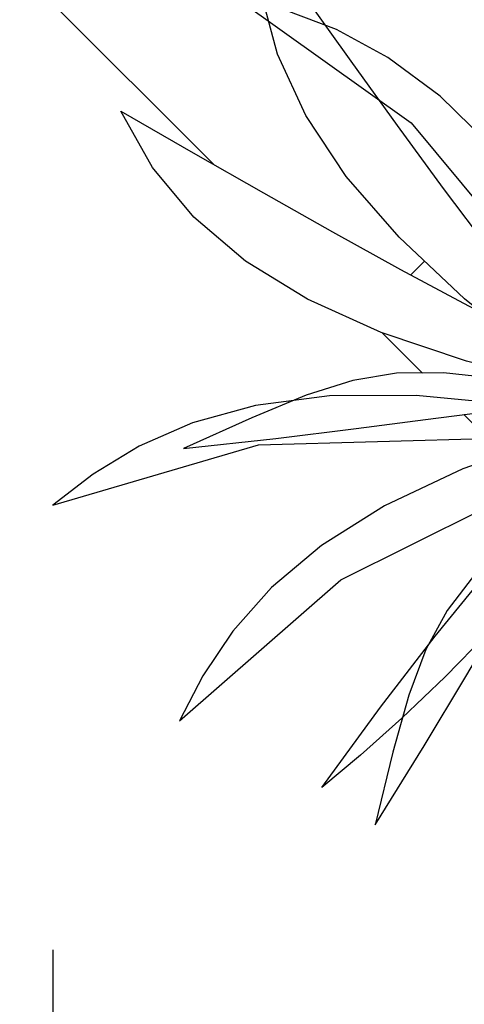
# Model space of a CAD drawing. Units: inches. Extents: x 3590 to 5167, y 65 to 1917.
# Tile 72 of 100: x 5035 to 5046, y 1765 to 1789. Entities that reach past the tile are written whole.
import ezdxf

# ---------------------------------------------------------------- set-up
doc = ezdxf.new("R2010")
doc.units = ezdxf.units.IN
for name, color, linetype, lineweight in [('A-ANNO-DIMS', 2, 'Continuous', 18), ('A-FLOR-PATT', 8, 'Continuous', 13), ('L-PLNT', 94, 'Continuous', 18)]:
    doc.layers.add(name, color=color, linetype=linetype, lineweight=lineweight)
doc.layers.add('DIENHOA', color=3, linetype='Continuous')
doc.styles.get("Standard").update_dxf_attribs({"font": 'arial.ttf'})
doc.dimstyles.new('ISO-25', dxfattribs={"dimtxt": 9, "dimasz": 2.5, "dimexe": 1.25, "dimexo": 0.625, "dimtad": 1, "dimdec": 1, "dimlunit": 3, "dimtxsty": 'Standard', "dimcen": 2.5, "dimadec": 0, "dimazin": 0, "dimtfac": 1, "dimtdec": 1, "dimtmove": 0, "dimatfit": 3, "dimfxl": 1, "dimarcsym": 0})

# ---------------------------------------------------------------- blocks, each defined once
blk = doc.blocks.new('Cay03_mb')
at = {"layer": 'DIENHOA'}
for p, q in [((-414.37, 402.78), (-240.22, 277.83)), ((-314.87, 371.26), (-365.2, 390.27)), ((-263.5, 343.48), (-314.87, 371.26)), ((-211.19, 304.6), (-263.5, 343.48)), ((-158.04, 252.34), (-211.19, 304.6)), ((-240.22, 277.83), (-88.39, 94.86)), ((-298.56, 20.07), (-345.02, 5.4)), ((-254.73, 27.37), (-298.56, 20.07)), ((-207.96, 27.76), (-254.73, 27.37)), ((-152.72, 21.72), (-207.96, 27.76)), ((-345.02, 5.4), (-399.63, -17.11)), ((-399.63, -17.11), (-467.96, -47.94)), ((-295.34, -27.91), (-225.83, -18.85)), ((-225.83, -18.85), (-165.8, -11.26)), ((-375.62, -37.81), (-295.34, -27.91)), ((-467.96, -47.94), (-375.62, -37.81)), ((-216.28, -235.58), (-165.86, -174.12)), ((-270.99, -306.55), (-216.28, -235.58)), ((-162.07, -230.91), (-206.29, -276.49)), ((-206.29, -276.49), (-249.56, -317.79)), ((-329.53, -387.1), (-270.99, -306.55)), ((-249.56, -317.79), (-290.96, -354.69)), ((-290.96, -354.69), (-329.53, -387.1))]:
    blk.add_line(p, q, dxfattribs=at)
for points in [[(-395.6, 473.65), (-347.51, 405.62), (-300.58, 339.5), (-254.33, 275.13), (-208.27, 212.32), (-161.92, 150.91), (-114.81, 90.72), (-66.46, 31.56), (-16.39, -26.73)], [(-16.39, -26.73), (-108.35, 38.55), (-186.88, 101.73), (-252.35, 163.45), (-305.09, 224.39), (-345.44, 285.22), (-373.75, 346.59), (-390.35, 409.18), (-395.6, 473.65)], [(-530.47, 289.69), (-458.27, 248.1), (-387.93, 207.77), (-318.94, 168.75), (-250.78, 131.06), (-182.94, 94.76), (-114.93, 59.88), (-46.22, 26.47), (23.69, -5.44)], [(23.69, -5.44), (-87.17, 15.25), (-184.97, 39.64), (-270.29, 68.2), (-343.73, 101.4), (-405.88, 139.68), (-457.33, 183.51), (-498.66, 233.36), (-530.47, 289.69)], [(-16.39, -26.73), (-133.98, -4.68), (-235.26, 5.29), (-321.98, 4.67), (-395.89, -5.03), (-458.73, -22.31), (-512.26, -45.67), (-558.22, -73.63), (-598.36, -104.66)], [(-471.89, -320.34), (-310.46, -179.32), (-97.66, -73.3), (23.69, -5.44)], [(23.69, -5.44), (-92.3, -34.76), (-188.42, -68.2), (-266.88, -105.14), (-329.9, -144.95), (-379.7, -187), (-418.48, -230.67), (-448.47, -275.32), (-471.89, -320.34)], [(-598.36, -104.66), (-392.67, -44.38), (-155.01, -37.42), (-16.39, -26.73)], [(-276.22, -424.43), (-227.35, -345.43), (-185.71, -276.08), (-150.05, -215.74), (-119.06, -163.76), (-91.49, -119.51), (-66.04, -82.35), (-41.43, -51.64), (-16.39, -26.73)], [(-16.39, -26.73), (-84.88, -85.96), (-136.99, -133.15), (-175.77, -172.96), (-204.26, -210.05), (-225.5, -249.08), (-242.55, -294.71), (-258.44, -351.61), (-276.22, -424.43)]]:
    blk.add_lwpolyline(points, dxfattribs=at)
blk = doc.blocks.new('*D322')
at = {"layer": 'A-ANNO-DIMS', "color": 0, "lineweight": -2, "transparency": 16777216}
for p, q in [((5035.744, 1766.184), (5035.744, 1761.199)), ((5064.812, 1766.184), (5064.812, 1761.199)), ((5038.244, 1762.449), (5062.312, 1762.449)), ((5064.812, 1762.449), (5166.991, 1762.449))]:
    blk.add_line(p, q, dxfattribs=at)
at = {"layer": 'A-ANNO-DIMS', "color": 0, "transparency": 16777216}
for points in [[(5038.244, 1762.866), (5038.244, 1762.032), (5035.744, 1762.449)], [(5062.312, 1762.866), (5062.312, 1762.032), (5064.812, 1762.449)]]:
    blk.add_solid(points, dxfattribs=at)
at = {"layer": 'Defpoints', "color": 0, "transparency": 16777216}
for p in [(5035.744, 1766.809), (5064.812, 1766.809), (5064.812, 1762.449)]:
    blk.add_point(p, dxfattribs=at)
at = {"layer": 'A-ANNO-DIMS', "color": 0, "transparency": 16777216, "insert": (5117.152, 1767.669), "char_height": 9, "attachment_point": 5}
blk.add_mtext('PLANT 2\'-5" TYP.', dxfattribs=at)
blk = doc.blocks.new('*D323')
at = {"layer": 'A-ANNO-DIMS', "color": 0, "lineweight": -2, "transparency": 16777216}
for p, q in [((5069.172, 1795.216), (5069.172, 1874.95)), ((5065.437, 1795.216), (5070.422, 1795.216)), ((5069.172, 1769.309), (5069.172, 1792.716)), ((5065.437, 1766.809), (5070.422, 1766.809))]:
    blk.add_line(p, q, dxfattribs=at)
at = {"layer": 'A-ANNO-DIMS', "color": 0, "transparency": 16777216}
for points in [[(5068.756, 1792.716), (5069.589, 1792.716), (5069.172, 1795.216)], [(5068.756, 1769.309), (5069.589, 1769.309), (5069.172, 1766.809)]]:
    blk.add_solid(points, dxfattribs=at)
at = {"layer": 'Defpoints', "color": 0, "transparency": 16777216}
for p in [(5064.812, 1795.216), (5069.172, 1795.216), (5064.812, 1766.809)]:
    blk.add_point(p, dxfattribs=at)
at = {"layer": 'A-ANNO-DIMS', "color": 0, "transparency": 16777216, "insert": (5063.894, 1836.333), "char_height": 9, "attachment_point": 5, "rotation": 90}
blk.add_mtext('2\'-4 1/2" TYP.', dxfattribs=at)

msp = doc.modelspace()

# ---------------------------------------------------------------- hatches: boundary and pattern name
at = {"layer": 'A-FLOR-PATT', "transparency": 33554687}
h = msp.add_hatch(dxfattribs=at)
h.set_pattern_fill('AR-HBONE', color=256, scale=0.2)
h.set_pattern_definition([(45, (-588.972, 0), (0, 28.73682), [60.96, -20.32]), (135, (-574.604, 14.368), (3e-15, 28.73682), [60.96, -20.32])])
h.paths.add_polyline_path([(5071.274, 1796.999), (4933.274, 1796.999), (4933.274, 1753.999), (4962.774, 1753.999, -0.414214), (4928.774, 1719.999), (4933.274, 1718.999), (4933.274, 1334.999), (5071.274, 1334.999)])
h.paths.add_polyline_path([(4951.78, 1521.077), (4951.715, 1521.04), (4951.563, 1520.895)], flags=16)
h.paths.add_polyline_path([(4952.267, 1521.376), (4952.198, 1521.371), (4952.198, 1521.356)], flags=0)
h.paths.add_polyline_path([(4967.051, 1529.728), (4965.231, 1528.694), (4963.411, 1527.714), (4961.756, 1526.851), (4963.589, 1527.449), (4964.036, 1527.478), (4962.975, 1527.249), (4961.76, 1526.852), (4959.792, 1525.834), (4958.005, 1524.895), (4956.24, 1523.93), (4954.504, 1522.919), (4954.129, 1522.682), (4953.361, 1521.997), (4953.366, 1521.998), (4953.605, 1522.064), (4955.106, 1522.761), (4956.921, 1523.434), (4958.678, 1523.915), (4960.358, 1524.2), (4961.945, 1524.286), (4964.171, 1524.108), (4965.958, 1523.309), (4963.863, 1522.976), (4965.187, 1522.499), (4963.366, 1522.497), (4961.545, 1522.487), (4959.764, 1522.461), (4958.304, 1522.419), (4957.974, 1522.388), (4956.307, 1522.232), (4954.718, 1522.071), (4953.251, 1521.899), (4953.525, 1521.623), (4954.331, 1521.379), (4956.243, 1521.23), (4958.039, 1520.93), (4959.684, 1520.483), (4961.16, 1519.896), (4963.107, 1518.8), (4964.393, 1517.325), (4962.973, 1517.726), (4964.558, 1516.661), (4965.407, 1515.708), (4963.507, 1516.322), (4961.68, 1517.005), (4959.935, 1517.745), (4958.282, 1518.528), (4956.732, 1519.343), (4955.295, 1520.175), (4954.672, 1520.572), (4954.513, 1520.627), (4955.658, 1519.318), (4956.703, 1517.982), (4957.644, 1516.647), (4958.485, 1515.334), (4959.55, 1513.524), (4960.438, 1511.769), (4958.841, 1513.62), (4957.452, 1515.325), (4955.819, 1517.459), (4956.665, 1515.448), (4957.111, 1513.923), (4957.447, 1511.714), (4957.076, 1509.793), (4956.538, 1511.11), (4955.992, 1512.569), (4955.444, 1514.125), (4954.898, 1515.735), (4954.357, 1517.356), (4953.824, 1518.943), (4953.305, 1520.452), (4953.065, 1521.116), (4952.971, 1521.146), (4952.949, 1521.086), (4952.73, 1520.199), (4953.37, 1518.024), (4953.757, 1516.373), (4954.051, 1514.765), (4954.264, 1513.221), (4954.471, 1511.131), (4954.497, 1510.402), (4954.409, 1511.76), (4954.264, 1513.221), (4954.051, 1514.765), (4953.757, 1516.373), (4953.37, 1518.024), (4952.877, 1519.698), (4952.716, 1520.141), (4952.533, 1519.059), (4952.374, 1517.789), (4952.219, 1516.312), (4952.046, 1514.6), (4951.833, 1512.626), (4951.557, 1510.363), (4951.203, 1512.168), (4950.852, 1514.339), (4950.985, 1516.376), (4951.66, 1518.286), (4952.593, 1520.481), (4952.357, 1521.13), (4951.855, 1520.328), (4950.839, 1518.908), (4949.777, 1517.587), (4948.916, 1516.617), (4948.111, 1515.256), (4947.089, 1513.554), (4945.889, 1511.615), (4946.326, 1513.402), (4946.562, 1514.249), (4945.528, 1513.327), (4944.581, 1512.531), (4946.018, 1514.508), (4947.204, 1516.048), (4947.893, 1517.313), (4949.307, 1518.764), (4950.414, 1519.767), (4950.451, 1519.806), (4952.267, 1521.376), (4951.645, 1521.493), (4950.404, 1521.18), (4948.044, 1520.359), (4946.119, 1519.452), (4944.572, 1518.475), (4943.35, 1517.443), (4941.997, 1515.92), (4941.661, 1515.275), (4942.813, 1516.99), (4944.572, 1518.475), (4946.119, 1519.452), (4948.044, 1520.359), (4950.404, 1521.18), (4951.645, 1521.493), (4949.647, 1521.868), (4948.6, 1521.756), (4947.126, 1521.57), (4945.42, 1521.348), (4943.45, 1521.105), (4941.183, 1520.856), (4942.86, 1521.613), (4943.873, 1522.03), (4942.952, 1521.909), (4941.41, 1521.485), (4939.543, 1520.67), (4938.968, 1520.226), (4940.733, 1521.299), (4942.952, 1521.909), (4943.702, 1522.008), (4945.894, 1522.7), (4947.565, 1522.714), (4948.921, 1522.566), (4951.131, 1522.183), (4950.971, 1522.297), (4948.129, 1523.006), (4946.035, 1523.707), (4944.232, 1524.521), (4942.707, 1525.461), (4941.444, 1526.537), (4940.43, 1527.761), (4939.649, 1529.143), (4941.421, 1528.122), (4943.147, 1527.132), (4944.841, 1526.175), (4946.514, 1525.25), (4948.179, 1524.359), (4948.365, 1524.263), (4946.475, 1526.045), (4945.181, 1527.54), (4944.19, 1529.033), (4943.496, 1530.54), (4943.278, 1531.36), (4942.498, 1531.919), (4943.114, 1531.762), (4942.959, 1533.659), (4944.14, 1531.989), (4944.612, 1531.323), (4946.202, 1530.463), (4947.486, 1529.509), (4948.79, 1528.226), (4950.368, 1526.237), (4949.485, 1528.155), (4948.851, 1530.123), (4948.491, 1532.041), (4948.381, 1533.918), (4948.501, 1535.76), (4948.827, 1537.573), (4949.418, 1535.565), (4949.957, 1533.569), (4950.464, 1531.586), (4950.961, 1529.617), (4951.391, 1527.954), (4951.724, 1530.687), (4952.201, 1532.58), (4952.889, 1534.33), (4953.77, 1535.951), (4954.827, 1537.46), (4954.521, 1535.39), (4954.273, 1533.937), (4955.58, 1535.663), (4956.748, 1536.739), (4956.159, 1534.78), (4955.589, 1532.873), (4955.043, 1531.006), (4954.525, 1529.166), (4954.038, 1527.341), (4953.638, 1525.733), (4953.611, 1525.586), (4953.398, 1524.166), (4953.382, 1524.009), (4954.07, 1525.476), (4954.912, 1527.022), (4956.136, 1528.894), (4957.847, 1530.577), (4959.376, 1531.54), (4958.256, 1530.104), (4957.143, 1528.663), (4956.066, 1527.243), (4955.056, 1525.871), (4954.141, 1524.571), (4953.352, 1523.372), (4953.311, 1523.303), (4953.273, 1522.925), (4953.261, 1522.382), (4954.103, 1523.373), (4954.63, 1524.284), (4955.961, 1526.358), (4957.23, 1528.13), (4958.421, 1529.609), (4960.037, 1531.368), (4961.374, 1532.375), (4962.101, 1532.77), (4961.07, 1531.061), (4959.987, 1529.438), (4958.869, 1527.908), (4958.15, 1527.007), (4959.803, 1528.003), (4961.589, 1528.793), (4963.391, 1529.328), (4965.211, 1529.632)], flags=16)
h.paths.add_polyline_path([(4962.944, 1523.182), (4961.107, 1523.422), (4960.392, 1523.362), (4962.35, 1523.331)], flags=0)
h.paths.add_polyline_path([(5049.541, 1584.551), (5049.476, 1584.515), (5049.325, 1584.37)], flags=16)
h.paths.add_polyline_path([(5050.028, 1584.851), (5049.959, 1584.845), (5049.959, 1584.83)], flags=0)
h.paths.add_polyline_path([(5042.333, 1581.949), (5043.88, 1582.926), (5045.806, 1583.833), (5048.165, 1584.654), (5049.406, 1584.967), (5047.408, 1585.342), (5046.361, 1585.231), (5044.888, 1585.044), (5043.181, 1584.822), (5041.211, 1584.579), (5038.944, 1584.33), (5040.622, 1585.087), (5041.634, 1585.504), (5040.713, 1585.383), (5039.171, 1584.959), (5037.304, 1584.144), (5036.729, 1583.7), (5038.494, 1584.773), (5040.713, 1585.383), (5041.463, 1585.482), (5043.655, 1586.174), (5045.326, 1586.188), (5046.682, 1586.04), (5048.893, 1585.657), (5048.732, 1585.771), (5045.891, 1586.48), (5043.796, 1587.181), (5041.994, 1587.996), (5040.468, 1588.935), (5039.205, 1590.011), (5038.191, 1591.235), (5037.41, 1592.617), (5039.182, 1591.596), (5040.909, 1590.607), (5042.602, 1589.649), (5044.275, 1588.724), (5045.94, 1587.833), (5046.126, 1587.738), (5044.237, 1589.519), (5042.942, 1591.015), (5041.952, 1592.508), (5041.257, 1594.014), (5041.039, 1594.834), (5040.26, 1595.393), (5040.875, 1595.237), (5040.721, 1597.133), (5041.901, 1595.463), (5042.373, 1594.798), (5043.963, 1593.938), (5045.247, 1592.983), (5046.552, 1591.701), (5048.129, 1589.712), (5047.247, 1591.63), (5046.613, 1593.597), (5046.252, 1595.515), (5046.142, 1597.392), (5046.262, 1599.234), (5046.588, 1601.047), (5047.179, 1599.039), (5047.718, 1597.043), (5048.225, 1595.06), (5048.722, 1593.091), (5049.152, 1591.429), (5049.485, 1594.161), (5049.962, 1596.054), (5050.65, 1597.804), (5051.532, 1599.425), (5052.589, 1600.934), (5052.283, 1598.864), (5052.034, 1597.411), (5053.341, 1599.137), (5054.509, 1600.213), (5053.92, 1598.254), (5053.35, 1596.348), (5052.805, 1594.48), (5052.286, 1592.64), (5051.799, 1590.815), (5051.4, 1589.207), (5051.373, 1589.06), (5051.159, 1587.64), (5051.143, 1587.483), (5051.831, 1588.95), (5052.673, 1590.496), (5053.898, 1592.368), (5055.608, 1594.051), (5057.137, 1595.014), (5056.017, 1593.578), (5054.904, 1592.137), (5053.828, 1590.717), (5052.817, 1589.345), (5051.902, 1588.046), (5051.113, 1586.846), (5051.072, 1586.777), (5051.034, 1586.399), (5051.022, 1585.856), (5051.864, 1586.847), (5052.391, 1587.758), (5053.723, 1589.832), (5054.991, 1591.604), (5056.182, 1593.083), (5057.798, 1594.842), (5059.135, 1595.849), (5059.863, 1596.244), (5058.831, 1594.535), (5057.749, 1592.912), (5056.63, 1591.382), (5055.912, 1590.482), (5057.564, 1591.477), (5059.35, 1592.267), (5061.152, 1592.802), (5062.972, 1593.106), (5064.812, 1593.203), (5062.992, 1592.169), (5061.172, 1591.188), (5059.518, 1590.325), (5061.35, 1590.924), (5061.797, 1590.952), (5060.737, 1590.723), (5059.521, 1590.326), (5057.553, 1589.308), (5055.766, 1588.369), (5054.002, 1587.404), (5052.265, 1586.393), (5051.891, 1586.156), (5051.122, 1585.471), (5051.127, 1585.472), (5051.366, 1585.538), (5052.867, 1586.235), (5054.682, 1586.908), (5056.439, 1587.389), (5058.12, 1587.675), (5059.706, 1587.76), (5061.933, 1587.583), (5063.719, 1586.783), (5061.624, 1586.45), (5062.949, 1585.973), (5061.127, 1585.971), (5059.307, 1585.961), (5057.525, 1585.935), (5056.065, 1585.893), (5055.735, 1585.862), (5054.068, 1585.707), (5052.479, 1585.546), (5051.012, 1585.373), (5051.286, 1585.097), (5052.092, 1584.853), (5054.004, 1584.704), (5055.8, 1584.404), (5057.446, 1583.958), (5058.921, 1583.37), (5060.868, 1582.274), (5062.154, 1580.799), (5060.734, 1581.2), (5062.32, 1580.135), (5063.168, 1579.182), (5061.269, 1579.796), (5059.441, 1580.479), (5057.696, 1581.219), (5056.043, 1582.003), (5054.493, 1582.817), (5053.057, 1583.649), (5052.433, 1584.047), (5052.274, 1584.101), (5053.42, 1582.793), (5054.464, 1581.457), (5055.405, 1580.121), (5056.247, 1578.809), (5057.311, 1576.998), (5058.199, 1575.244), (5056.602, 1577.094), (5055.213, 1578.799), (5053.58, 1580.933), (5054.427, 1578.922), (5054.872, 1577.397), (5055.208, 1575.189), (5054.838, 1573.267), (5054.299, 1574.584), (5053.754, 1576.043), (5053.206, 1577.599), (5052.659, 1579.209), (5052.118, 1580.83), (5051.585, 1582.417), (5051.066, 1583.927), (5050.826, 1584.59), (5050.733, 1584.62), (5050.711, 1584.561), (5050.491, 1583.673), (5051.131, 1581.498), (5051.518, 1579.847), (5051.813, 1578.24), (5052.026, 1576.695), (5052.233, 1574.605), (5052.258, 1573.876), (5052.17, 1575.234), (5052.026, 1576.695), (5051.813, 1578.24), (5051.518, 1579.847), (5051.131, 1581.498), (5050.638, 1583.172), (5050.477, 1583.615), (5050.294, 1582.533), (5050.136, 1581.263), (5049.981, 1579.786), (5049.807, 1578.074), (5049.594, 1576.1), (5049.318, 1573.837), (5048.965, 1575.642), (5048.613, 1577.813), (5048.747, 1579.85), (5049.421, 1581.76), (5050.354, 1583.955), (5050.118, 1584.604), (5049.616, 1583.802), (5048.6, 1582.382), (5047.538, 1581.061), (5046.677, 1580.091), (5045.872, 1578.73), (5044.85, 1577.028), (5043.651, 1575.089), (5044.087, 1576.877), (5044.324, 1577.723), (5043.289, 1576.801), (5042.342, 1576.005), (5043.779, 1577.982), (5044.966, 1579.522), (5045.655, 1580.787), (5047.068, 1582.239), (5048.175, 1583.241), (5048.213, 1583.28), (5050.028, 1584.851), (5049.406, 1584.967), (5048.165, 1584.654), (5045.806, 1583.833), (5043.88, 1582.926), (5042.333, 1581.949), (5041.111, 1580.917), (5039.758, 1579.394), (5039.423, 1578.749), (5040.575, 1580.464)], flags=16)
h.paths.add_polyline_path([(4954.799, 1533.12), (4954.262, 1532.079), (4953.831, 1530.935), (4953.505, 1529.636), (4953.283, 1528.133), (4953.167, 1526.376), (4953.156, 1524.315), (4953.277, 1521.236), (4952.802, 1521.842), (4951.557, 1521.998), (4950.976, 1521.961), (4952.661, 1521.941), (4952.802, 1521.842), (4953.152, 1523.593), (4953.167, 1526.376), (4953.283, 1528.133), (4953.609, 1530.346), (4954.456, 1532.592)], flags=0)
h.paths.add_polyline_path([(5050.563, 1585.316), (5049.318, 1585.472), (5048.737, 1585.435), (5050.422, 1585.415), (5050.563, 1585.316), (5050.914, 1587.067), (5050.928, 1589.851), (5051.045, 1591.607), (5051.371, 1593.82), (5052.217, 1596.066), (5052.56, 1596.594), (5052.024, 1595.554), (5051.592, 1594.409), (5051.266, 1593.11), (5051.045, 1591.607), (5050.928, 1589.851), (5050.918, 1587.789), (5051.038, 1584.71)], flags=0)
h.paths.add_polyline_path([(5058.153, 1586.836), (5060.111, 1586.805), (5060.705, 1586.656), (5058.868, 1586.896)], flags=0)
h.paths.add_polyline_path([(5049.541, 1430.936), (5049.476, 1430.9), (5049.325, 1430.755)], flags=16)
h.paths.add_polyline_path([(5050.028, 1431.236), (5049.959, 1431.231), (5049.959, 1431.215)], flags=0)
h.paths.add_polyline_path([(5046.588, 1447.432), (5047.179, 1445.425), (5047.718, 1443.429), (5048.225, 1441.446), (5048.722, 1439.476), (5049.152, 1437.814), (5049.485, 1440.546), (5049.962, 1442.439), (5050.65, 1444.189), (5051.532, 1445.811), (5052.589, 1447.319), (5052.283, 1445.249), (5052.034, 1443.796), (5053.341, 1445.522), (5054.509, 1446.598), (5053.92, 1444.64), (5053.35, 1442.733), (5052.805, 1440.865), (5052.286, 1439.025), (5051.799, 1437.201), (5051.4, 1435.592), (5051.373, 1435.445), (5051.159, 1434.025), (5051.143, 1433.868), (5051.831, 1435.335), (5052.673, 1436.881), (5053.898, 1438.753), (5055.608, 1440.436), (5057.137, 1441.4), (5056.017, 1439.963), (5054.904, 1438.522), (5053.828, 1437.102), (5052.817, 1435.73), (5051.902, 1434.431), (5051.113, 1433.231), (5051.072, 1433.162), (5051.034, 1432.784), (5051.022, 1432.242), (5051.864, 1433.232), (5052.391, 1434.143), (5053.723, 1436.217), (5054.991, 1437.989), (5056.182, 1439.468), (5057.798, 1441.227), (5059.135, 1442.235), (5059.863, 1442.629), (5058.831, 1440.921), (5057.749, 1439.298), (5056.63, 1437.767), (5055.912, 1436.867), (5057.564, 1437.863), (5059.35, 1438.652), (5061.152, 1439.187), (5062.972, 1439.491), (5064.812, 1439.588), (5062.992, 1438.554), (5061.172, 1437.573), (5059.518, 1436.71), (5061.35, 1437.309), (5061.797, 1437.337), (5060.737, 1437.108), (5059.521, 1436.711), (5057.553, 1435.693), (5055.766, 1434.754), (5054.002, 1433.789), (5052.265, 1432.778), (5051.891, 1432.541), (5051.122, 1431.856), (5051.127, 1431.857), (5051.366, 1431.923), (5052.867, 1432.62), (5054.682, 1433.293), (5056.439, 1433.775), (5058.12, 1434.06), (5059.706, 1434.145), (5061.933, 1433.968), (5063.719, 1433.168), (5061.624, 1432.835), (5062.949, 1432.358), (5061.127, 1432.357), (5059.307, 1432.346), (5057.525, 1432.32), (5056.065, 1432.278), (5055.735, 1432.248), (5054.068, 1432.092), (5052.479, 1431.931), (5051.012, 1431.759), (5051.286, 1431.482), (5052.092, 1431.238), (5054.004, 1431.089), (5055.8, 1430.789), (5057.446, 1430.343), (5058.921, 1429.755), (5060.868, 1428.66), (5062.154, 1427.185), (5060.734, 1427.585), (5062.32, 1426.52), (5063.168, 1425.567), (5061.269, 1426.181), (5059.441, 1426.865), (5057.696, 1427.604), (5056.043, 1428.388), (5054.493, 1429.202), (5053.057, 1430.034), (5052.433, 1430.432), (5052.274, 1430.487), (5053.42, 1429.178), (5054.464, 1427.842), (5055.405, 1426.506), (5056.247, 1425.194), (5057.311, 1423.383), (5058.199, 1421.629), (5056.602, 1423.479), (5055.213, 1425.184), (5053.58, 1427.318), (5054.427, 1425.307), (5054.872, 1423.782), (5055.208, 1421.574), (5054.838, 1419.652), (5054.299, 1420.97), (5053.754, 1422.428), (5053.206, 1423.984), (5052.659, 1425.595), (5052.118, 1427.215), (5051.585, 1428.802), (5051.066, 1430.312), (5050.826, 1430.975), (5050.733, 1431.005), (5050.711, 1430.946), (5050.491, 1430.058), (5051.131, 1427.883), (5051.518, 1426.232), (5051.813, 1424.625), (5052.026, 1423.081), (5052.233, 1420.991), (5052.258, 1420.261), (5052.17, 1421.619), (5052.026, 1423.081), (5051.813, 1424.625), (5051.518, 1426.232), (5051.131, 1427.883), (5050.638, 1429.558), (5050.477, 1430.001), (5050.294, 1428.918), (5050.136, 1427.648), (5049.981, 1426.171), (5049.807, 1424.459), (5049.594, 1422.485), (5049.318, 1420.222), (5048.965, 1422.028), (5048.613, 1424.199), (5048.747, 1426.235), (5049.421, 1428.146), (5050.354, 1430.34), (5050.118, 1430.989), (5049.616, 1430.187), (5048.6, 1428.768), (5047.538, 1427.446), (5046.677, 1426.477), (5045.872, 1425.116), (5044.85, 1423.413), (5043.651, 1421.474), (5044.087, 1423.262), (5044.324, 1424.109), (5043.289, 1423.186), (5042.342, 1422.391), (5043.779, 1424.368), (5044.966, 1425.907), (5045.655, 1427.173), (5047.068, 1428.624), (5048.175, 1429.627), (5048.213, 1429.666), (5050.028, 1431.236), (5049.406, 1431.353), (5048.165, 1431.039), (5045.806, 1430.218), (5043.88, 1429.311), (5042.333, 1428.334), (5041.111, 1427.302), (5039.758, 1425.779), (5039.423, 1425.134), (5040.575, 1426.849), (5042.333, 1428.334), (5043.88, 1429.311), (5045.806, 1430.218), (5048.165, 1431.039), (5049.406, 1431.353), (5047.408, 1431.727), (5046.361, 1431.616), (5044.888, 1431.429), (5043.181, 1431.207), (5041.211, 1430.964), (5038.944, 1430.715), (5040.622, 1431.472), (5041.634, 1431.89), (5040.713, 1431.769), (5039.171, 1431.345), (5037.304, 1430.53), (5036.729, 1430.085), (5038.494, 1431.158), (5040.713, 1431.769), (5041.463, 1431.867), (5043.655, 1432.559), (5045.326, 1432.573), (5046.682, 1432.425), (5048.893, 1432.042), (5048.732, 1432.156), (5045.891, 1432.865), (5043.796, 1433.566), (5041.994, 1434.381), (5040.468, 1435.321), (5039.205, 1436.396), (5038.191, 1437.62), (5037.41, 1439.002), (5039.182, 1437.982), (5040.909, 1436.992), (5042.602, 1436.034), (5044.275, 1435.109), (5045.94, 1434.218), (5046.126, 1434.123), (5044.237, 1435.904), (5042.942, 1437.4), (5041.952, 1438.893), (5041.257, 1440.399), (5041.039, 1441.219), (5040.26, 1441.778), (5040.875, 1441.622), (5040.721, 1443.518), (5041.901, 1441.848), (5042.373, 1441.183), (5043.963, 1440.323), (5045.247, 1439.369), (5046.552, 1438.086), (5048.129, 1436.097), (5047.247, 1438.015), (5046.613, 1439.982), (5046.252, 1441.901), (5046.142, 1443.778), (5046.262, 1445.619)], flags=16)
h.paths.add_polyline_path([(5052.382, 1444.255), (5051.623, 1442.78), (5052.024, 1441.939), (5052.56, 1442.98)], flags=0)
h.paths.add_polyline_path([(5050.563, 1431.701), (5049.318, 1431.857), (5048.737, 1431.821), (5050.422, 1431.8)], flags=0)
h.paths.add_polyline_path([(5058.153, 1433.221), (5060.111, 1433.19), (5060.705, 1433.041), (5058.868, 1433.281)], flags=0)
h.paths.add_polyline_path([(5049.541, 1352.285), (5049.476, 1352.249), (5049.325, 1352.104)], flags=16)
h.paths.add_polyline_path([(5050.028, 1352.585), (5049.959, 1352.58), (5049.959, 1352.564)], flags=0)
h.paths.add_polyline_path([(5046.588, 1368.781), (5047.179, 1366.774), (5047.718, 1364.778), (5048.225, 1362.795), (5048.722, 1360.825), (5049.152, 1359.163), (5049.485, 1361.896), (5049.962, 1363.789), (5050.65, 1365.538), (5051.532, 1367.16), (5052.589, 1368.669), (5052.283, 1366.598), (5052.034, 1365.145), (5053.341, 1366.871), (5054.509, 1367.947), (5053.92, 1365.989), (5053.35, 1364.082), (5052.805, 1362.214), (5052.286, 1360.374), (5051.799, 1358.55), (5051.4, 1356.942), (5051.373, 1356.794), (5051.159, 1355.374), (5051.143, 1355.218), (5051.831, 1356.684), (5052.673, 1358.23), (5053.898, 1360.102), (5055.608, 1361.786), (5057.137, 1362.749), (5056.017, 1361.313), (5054.904, 1359.872), (5053.828, 1358.452), (5052.817, 1357.079), (5051.902, 1355.78), (5051.113, 1354.581), (5051.072, 1354.512), (5051.034, 1354.133), (5051.022, 1353.591), (5051.864, 1354.581), (5052.391, 1355.492), (5053.723, 1357.566), (5054.991, 1359.338), (5056.182, 1360.817), (5057.798, 1362.577), (5059.135, 1363.584), (5059.863, 1363.979), (5058.831, 1362.27), (5057.749, 1360.647), (5056.63, 1359.117), (5055.912, 1358.216), (5057.564, 1359.212), (5059.35, 1360.001), (5061.152, 1360.536), (5062.972, 1360.841), (5064.812, 1360.937), (5062.992, 1359.903), (5061.172, 1358.923), (5059.518, 1358.059), (5061.35, 1358.658), (5061.797, 1358.687), (5060.737, 1358.458), (5059.521, 1358.061), (5057.553, 1357.043), (5055.766, 1356.103), (5054.002, 1355.138), (5052.265, 1354.127), (5051.891, 1353.89), (5051.122, 1353.206), (5051.127, 1353.206), (5051.366, 1353.272), (5052.867, 1353.969), (5054.682, 1354.643), (5056.439, 1355.124), (5058.12, 1355.409), (5059.706, 1355.495), (5061.933, 1355.317), (5063.719, 1354.518), (5061.624, 1354.184), (5062.949, 1353.708), (5061.127, 1353.706), (5059.307, 1353.695), (5057.525, 1353.669), (5056.065, 1353.627), (5055.735, 1353.597), (5054.068, 1353.441), (5052.479, 1353.28), (5051.012, 1353.108), (5051.286, 1352.831), (5052.092, 1352.587), (5054.004, 1352.439), (5055.8, 1352.138), (5057.446, 1351.692), (5058.921, 1351.104), (5060.868, 1350.009), (5062.154, 1348.534), (5060.734, 1348.935), (5062.32, 1347.869), (5063.168, 1346.916), (5061.269, 1347.53), (5059.441, 1348.214), (5057.696, 1348.954), (5056.043, 1349.737), (5054.493, 1350.551), (5053.057, 1351.383), (5052.433, 1351.781), (5052.274, 1351.836), (5053.42, 1350.527), (5054.464, 1349.191), (5055.405, 1347.855), (5056.247, 1346.543), (5057.311, 1344.733), (5058.199, 1342.978), (5056.602, 1344.828), (5055.213, 1346.534), (5053.58, 1348.667), (5054.427, 1346.656), (5054.872, 1345.132), (5055.208, 1342.923), (5054.838, 1341.002), (5054.299, 1342.319), (5053.754, 1343.778), (5053.206, 1345.334), (5052.659, 1346.944), (5052.118, 1348.564), (5051.585, 1350.151), (5051.066, 1351.661), (5050.826, 1352.324), (5050.733, 1352.355), (5050.711, 1352.295), (5050.491, 1351.408), (5051.131, 1349.232), (5051.518, 1347.581), (5051.813, 1345.974), (5052.026, 1344.43), (5052.233, 1342.34), (5052.258, 1341.61), (5052.17, 1342.969), (5052.026, 1344.43), (5051.813, 1345.974), (5051.518, 1347.581), (5051.131, 1349.232), (5050.638, 1350.907), (5050.477, 1351.35), (5050.294, 1350.267), (5050.136, 1348.997), (5049.981, 1347.52), (5049.807, 1345.809), (5049.594, 1343.835), (5049.318, 1341.571), (5048.965, 1343.377), (5048.613, 1345.548), (5048.747, 1347.585), (5049.421, 1349.495), (5050.354, 1351.689), (5050.118, 1352.339), (5049.616, 1351.536), (5048.6, 1350.117), (5047.538, 1348.795), (5046.677, 1347.826), (5045.872, 1346.465), (5044.85, 1344.763), (5043.651, 1342.824), (5044.087, 1344.611), (5044.324, 1345.458), (5043.289, 1344.535), (5042.342, 1343.74), (5043.779, 1345.717), (5044.966, 1347.256), (5045.655, 1348.522), (5047.068, 1349.973), (5048.175, 1350.976), (5048.213, 1351.015), (5050.028, 1352.585), (5049.406, 1352.702), (5048.165, 1352.388), (5045.806, 1351.567), (5043.88, 1350.661), (5042.333, 1349.683), (5041.111, 1348.651), (5039.758, 1347.128), (5039.423, 1346.483), (5040.575, 1348.198), (5042.333, 1349.683), (5043.88, 1350.661), (5045.806, 1351.567), (5048.165, 1352.388), (5049.406, 1352.702), (5047.408, 1353.076), (5046.361, 1352.965), (5044.888, 1352.779), (5043.181, 1352.556), (5041.211, 1352.313), (5038.944, 1352.065), (5040.622, 1352.821), (5041.634, 1353.239), (5040.713, 1353.118), (5039.171, 1352.694), (5037.304, 1351.879), (5036.729, 1351.434), (5038.494, 1352.508), (5040.713, 1353.118), (5041.463, 1353.216), (5043.655, 1353.909), (5045.326, 1353.923), (5046.682, 1353.774), (5048.893, 1353.391), (5048.732, 1353.506), (5045.891, 1354.214), (5043.796, 1354.915), (5041.994, 1355.73), (5040.468, 1356.67), (5039.205, 1357.746), (5038.191, 1358.969), (5037.41, 1360.352), (5039.182, 1359.331), (5040.909, 1358.341), (5042.602, 1357.383), (5044.275, 1356.458), (5045.94, 1355.567), (5046.126, 1355.472), (5044.237, 1357.253), (5042.942, 1358.749), (5041.952, 1360.242), (5041.257, 1361.748), (5041.039, 1362.568), (5040.26, 1363.128), (5040.875, 1362.971), (5040.721, 1364.867), (5041.901, 1363.197), (5042.373, 1362.532), (5043.963, 1361.672), (5045.247, 1360.718), (5046.552, 1359.435), (5048.129, 1357.446), (5047.247, 1359.364), (5046.613, 1361.331), (5046.252, 1363.25), (5046.142, 1365.127), (5046.262, 1366.969)], flags=16)
h.paths.add_polyline_path([(5052.382, 1365.604), (5051.623, 1364.129), (5052.024, 1363.288), (5052.56, 1364.329)], flags=0)
h.paths.add_polyline_path([(4951.78, 1698.041), (4951.715, 1698.005), (4951.563, 1697.859)], flags=16)
h.paths.add_polyline_path([(4952.267, 1698.341), (4952.198, 1698.335), (4952.198, 1698.32)], flags=0)
h.paths.add_polyline_path([(4957.076, 1686.757), (4956.538, 1688.074), (4955.992, 1689.533), (4955.444, 1691.089), (4954.898, 1692.699), (4954.357, 1694.32), (4953.824, 1695.907), (4953.305, 1697.417), (4953.065, 1698.08), (4952.971, 1698.11), (4952.949, 1698.051), (4952.73, 1697.163), (4953.37, 1694.988), (4953.757, 1693.337), (4954.051, 1691.729), (4954.264, 1690.185), (4954.471, 1688.095), (4954.497, 1687.366), (4954.409, 1688.724), (4954.264, 1690.185), (4954.051, 1691.729), (4953.757, 1693.337), (4953.37, 1694.988), (4952.877, 1696.662), (4952.716, 1697.105), (4952.533, 1696.023), (4952.374, 1694.753), (4952.219, 1693.276), (4952.046, 1691.564), (4951.833, 1689.59), (4951.557, 1687.327), (4951.203, 1689.132), (4950.852, 1691.303), (4950.985, 1693.34), (4951.66, 1695.25), (4952.593, 1697.445), (4952.357, 1698.094), (4951.855, 1697.292), (4950.839, 1695.872), (4949.777, 1694.551), (4948.916, 1693.581), (4948.111, 1692.22), (4947.089, 1690.518), (4945.889, 1688.579), (4946.326, 1690.366), (4946.562, 1691.213), (4945.528, 1690.291), (4944.581, 1689.495), (4946.018, 1691.472), (4947.204, 1693.012), (4947.893, 1694.277), (4949.307, 1695.729), (4950.414, 1696.731), (4950.451, 1696.77), (4952.267, 1698.341), (4951.645, 1698.457), (4950.404, 1698.144), (4948.044, 1697.323), (4946.119, 1696.416), (4944.572, 1695.439), (4943.35, 1694.407), (4941.997, 1692.884), (4941.661, 1692.239), (4942.813, 1693.954), (4944.572, 1695.439), (4946.119, 1696.416), (4948.044, 1697.323), (4950.404, 1698.144), (4951.645, 1698.457), (4949.647, 1698.832), (4948.6, 1698.72), (4947.126, 1698.534), (4945.42, 1698.312), (4943.45, 1698.069), (4941.183, 1697.82), (4942.86, 1698.577), (4943.873, 1698.994), (4942.952, 1698.873), (4941.41, 1698.449), (4939.543, 1697.634), (4938.968, 1697.19), (4940.733, 1698.263), (4942.952, 1698.873), (4943.702, 1698.972), (4945.894, 1699.664), (4947.565, 1699.678), (4948.921, 1699.53), (4951.131, 1699.147), (4950.971, 1699.261), (4948.129, 1699.97), (4946.035, 1700.671), (4944.232, 1701.486), (4942.707, 1702.425), (4941.444, 1703.501), (4940.43, 1704.725), (4939.649, 1706.107), (4941.421, 1705.086), (4943.147, 1704.097), (4944.841, 1703.139), (4946.514, 1702.214), (4948.179, 1701.323), (4948.365, 1701.227), (4946.475, 1703.009), (4945.181, 1704.505), (4944.19, 1705.997), (4943.496, 1707.504), (4943.278, 1708.324), (4942.498, 1708.883), (4943.114, 1708.727), (4942.959, 1710.623), (4944.14, 1708.953), (4944.612, 1708.287), (4946.202, 1707.428), (4947.486, 1706.473), (4948.79, 1705.191), (4950.368, 1703.202), (4949.485, 1705.12), (4948.851, 1707.087), (4948.491, 1709.005), (4948.381, 1710.882), (4948.501, 1712.724), (4948.827, 1714.537), (4949.418, 1712.529), (4949.957, 1710.533), (4950.464, 1708.55), (4950.961, 1706.581), (4951.391, 1704.919), (4951.724, 1707.651), (4952.201, 1709.544), (4952.889, 1711.294), (4953.77, 1712.915), (4954.827, 1714.424), (4954.521, 1712.354), (4954.273, 1710.901), (4955.58, 1712.627), (4956.748, 1713.703), (4956.159, 1711.744), (4955.589, 1709.837), (4955.043, 1707.97), (4954.525, 1706.13), (4954.038, 1704.305), (4953.638, 1702.697), (4953.611, 1702.55), (4953.398, 1701.13), (4953.382, 1700.973), (4954.07, 1702.44), (4954.912, 1703.986), (4956.136, 1705.858), (4957.847, 1707.541), (4959.376, 1708.504), (4958.256, 1707.068), (4957.143, 1705.627), (4956.066, 1704.207), (4955.056, 1702.835), (4954.141, 1701.536), (4953.352, 1700.336), (4953.311, 1700.267), (4953.273, 1699.889), (4953.261, 1699.346), (4954.103, 1700.337), (4954.63, 1701.248), (4955.961, 1703.322), (4957.23, 1705.094), (4958.421, 1706.573), (4960.037, 1708.332), (4961.374, 1709.339), (4962.101, 1709.734), (4961.07, 1708.025), (4959.987, 1706.402), (4958.869, 1704.872), (4958.15, 1703.972), (4959.803, 1704.967), (4961.589, 1705.757), (4963.391, 1706.292), (4965.211, 1706.596), (4967.051, 1706.692), (4965.231, 1705.659), (4963.411, 1704.678), (4961.756, 1703.815), (4963.589, 1704.413), (4964.036, 1704.442), (4962.975, 1704.213), (4961.76, 1703.816), (4959.792, 1702.798), (4958.005, 1701.859), (4956.24, 1700.894), (4954.504, 1699.883), (4954.129, 1699.646), (4953.361, 1698.961), (4953.366, 1698.962), (4953.605, 1699.028), (4955.106, 1699.725), (4956.921, 1700.398), (4958.678, 1700.879), (4960.358, 1701.164), (4961.945, 1701.25), (4964.171, 1701.073), (4965.958, 1700.273), (4963.863, 1699.94), (4965.187, 1699.463), (4963.366, 1699.461), (4961.545, 1699.451), (4959.764, 1699.425), (4958.304, 1699.383), (4957.974, 1699.352), (4956.307, 1699.197), (4954.718, 1699.036), (4953.251, 1698.863), (4953.525, 1698.587), (4954.331, 1698.343), (4956.243, 1698.194), (4958.039, 1697.894), (4959.684, 1697.447), (4961.16, 1696.86), (4963.107, 1695.764), (4964.393, 1694.289), (4962.973, 1694.69), (4964.558, 1693.625), (4965.407, 1692.672), (4963.507, 1693.286), (4961.68, 1693.969), (4959.935, 1694.709), (4958.282, 1695.492), (4956.732, 1696.307), (4955.295, 1697.139), (4954.672, 1697.536), (4954.513, 1697.591), (4955.658, 1696.282), (4956.703, 1694.946), (4957.644, 1693.611), (4958.485, 1692.298), (4959.55, 1690.488), (4960.438, 1688.733), (4958.841, 1690.584), (4957.452, 1692.289), (4955.819, 1694.423), (4956.665, 1692.412), (4957.111, 1690.887), (4957.447, 1688.678)], flags=16)
h.paths.add_polyline_path([(5050.563, 1353.05), (5049.318, 1353.207), (5048.737, 1353.17), (5050.422, 1353.15)], flags=0)
h.paths.add_polyline_path([(4951.78, 1351.486), (4951.715, 1351.45), (4951.563, 1351.305)], flags=16)
h.paths.add_polyline_path([(4952.267, 1351.786), (4952.198, 1351.78), (4952.198, 1351.765)], flags=0)
h.paths.add_polyline_path([(4954.827, 1367.869), (4954.521, 1365.799), (4954.273, 1364.346), (4955.58, 1366.072), (4956.748, 1367.148), (4956.159, 1365.19), (4955.589, 1363.283), (4955.043, 1361.415), (4954.525, 1359.575), (4954.038, 1357.751), (4953.638, 1356.142), (4953.611, 1355.995), (4953.398, 1354.575), (4953.382, 1354.418), (4954.07, 1355.885), (4954.912, 1357.431), (4956.136, 1359.303), (4957.847, 1360.986), (4959.376, 1361.95), (4958.256, 1360.513), (4957.143, 1359.072), (4956.066, 1357.652), (4955.056, 1356.28), (4954.141, 1354.981), (4953.352, 1353.781), (4953.311, 1353.712), (4953.273, 1353.334), (4953.261, 1352.792), (4954.103, 1353.782), (4954.63, 1354.693), (4955.961, 1356.767), (4957.23, 1358.539), (4958.421, 1360.018), (4960.037, 1361.777), (4961.374, 1362.785), (4962.101, 1363.179), (4961.07, 1361.471), (4959.987, 1359.848), (4958.869, 1358.317), (4958.15, 1357.417), (4959.803, 1358.413), (4961.589, 1359.202), (4963.391, 1359.737), (4965.211, 1360.041), (4967.051, 1360.138), (4965.231, 1359.104), (4963.411, 1358.123), (4961.756, 1357.26), (4963.589, 1357.859), (4964.036, 1357.887), (4962.975, 1357.658), (4961.76, 1357.261), (4959.792, 1356.243), (4958.005, 1355.304), (4956.24, 1354.339), (4954.504, 1353.328), (4954.129, 1353.091), (4953.361, 1352.406), (4953.366, 1352.407), (4953.605, 1352.473), (4955.106, 1353.17), (4956.921, 1353.843), (4958.678, 1354.325), (4960.358, 1354.61), (4961.945, 1354.695), (4964.171, 1354.518), (4965.958, 1353.718), (4963.863, 1353.385), (4965.187, 1352.908), (4963.366, 1352.907), (4961.545, 1352.896), (4959.764, 1352.87), (4958.304, 1352.828), (4957.974, 1352.798), (4956.307, 1352.642), (4954.718, 1352.481), (4953.251, 1352.309), (4953.525, 1352.032), (4954.331, 1351.788), (4956.243, 1351.639), (4958.039, 1351.339), (4959.684, 1350.893), (4961.16, 1350.305), (4963.107, 1349.21), (4964.393, 1347.735), (4962.973, 1348.135), (4964.558, 1347.07), (4965.407, 1346.117), (4963.507, 1346.731), (4961.68, 1347.414), (4959.935, 1348.154), (4958.282, 1348.938), (4956.732, 1349.752), (4955.295, 1350.584), (4954.672, 1350.982), (4954.513, 1351.036), (4955.658, 1349.728), (4956.703, 1348.392), (4957.644, 1347.056), (4958.485, 1345.744), (4959.55, 1343.933), (4960.438, 1342.179), (4958.841, 1344.029), (4957.452, 1345.734), (4955.819, 1347.868), (4956.665, 1345.857), (4957.111, 1344.332), (4957.447, 1342.124), (4957.076, 1340.202), (4956.538, 1341.52), (4955.992, 1342.978), (4955.444, 1344.534), (4954.898, 1346.145), (4954.357, 1347.765), (4953.824, 1349.352), (4953.305, 1350.862), (4953.065, 1351.525), (4952.971, 1351.555), (4952.949, 1351.496), (4952.73, 1350.608), (4953.37, 1348.433), (4953.757, 1346.782), (4954.051, 1345.175), (4954.264, 1343.631), (4954.471, 1341.541), (4954.497, 1340.811), (4954.409, 1342.169), (4954.264, 1343.631), (4954.051, 1345.175), (4953.757, 1346.782), (4953.37, 1348.433), (4952.877, 1350.108), (4952.716, 1350.551), (4952.533, 1349.468), (4952.374, 1348.198), (4952.219, 1346.721), (4952.046, 1345.009), (4951.833, 1343.035), (4951.557, 1340.772), (4951.203, 1342.578), (4950.852, 1344.749), (4950.985, 1346.785), (4951.66, 1348.696), (4952.593, 1350.89), (4952.357, 1351.539), (4951.855, 1350.737), (4950.839, 1349.318), (4949.777, 1347.996), (4948.916, 1347.027), (4948.111, 1345.665), (4947.089, 1343.963), (4945.889, 1342.024), (4946.326, 1343.812), (4946.562, 1344.659), (4945.528, 1343.736), (4944.581, 1342.941), (4946.018, 1344.918), (4947.204, 1346.457), (4947.893, 1347.723), (4949.307, 1349.174), (4950.414, 1350.177), (4950.451, 1350.216), (4952.267, 1351.786), (4951.645, 1351.903), (4950.404, 1351.589), (4948.044, 1350.768), (4946.119, 1349.861), (4944.572, 1348.884), (4943.35, 1347.852), (4941.997, 1346.329), (4941.661, 1345.684), (4942.813, 1347.399), (4944.572, 1348.884), (4946.119, 1349.861), (4948.044, 1350.768), (4950.404, 1351.589), (4951.645, 1351.903), (4949.647, 1352.277), (4948.6, 1352.166), (4947.126, 1351.979), (4945.42, 1351.757), (4943.45, 1351.514), (4941.183, 1351.265), (4942.86, 1352.022), (4943.873, 1352.44), (4942.952, 1352.319), (4941.41, 1351.895), (4939.543, 1351.08), (4938.968, 1350.635), (4940.733, 1351.708), (4942.952, 1352.319), (4943.702, 1352.417), (4945.894, 1353.109), (4947.565, 1353.123), (4948.921, 1352.975), (4951.131, 1352.592), (4950.971, 1352.706), (4948.129, 1353.415), (4946.035, 1354.116), (4944.232, 1354.931), (4942.707, 1355.871), (4941.444, 1356.946), (4940.43, 1358.17), (4939.649, 1359.552), (4941.421, 1358.532), (4943.147, 1357.542), (4944.841, 1356.584), (4946.514, 1355.659), (4948.179, 1354.768), (4948.365, 1354.673), (4946.475, 1356.454), (4945.181, 1357.95), (4944.19, 1359.443), (4943.496, 1360.949), (4943.278, 1361.769), (4942.498, 1362.328), (4943.114, 1362.172), (4942.959, 1364.068), (4944.14, 1362.398), (4944.612, 1361.733), (4946.202, 1360.873), (4947.486, 1359.919), (4948.79, 1358.636), (4950.368, 1356.647), (4949.485, 1358.565), (4948.851, 1360.532), (4948.491, 1362.451), (4948.381, 1364.328), (4948.501, 1366.169), (4948.827, 1367.982), (4949.418, 1365.975), (4949.957, 1363.979), (4950.464, 1361.995), (4950.961, 1360.026), (4951.391, 1358.364), (4951.724, 1361.096), (4952.201, 1362.989), (4952.889, 1364.739), (4953.77, 1366.361)], flags=16)
h.paths.add_polyline_path([(4954.799, 1363.53), (4954.262, 1362.489), (4953.831, 1361.344), (4953.505, 1360.045), (4953.283, 1358.543), (4953.167, 1356.786), (4953.156, 1354.724), (4953.277, 1351.646), (4952.802, 1352.251), (4951.557, 1352.407), (4950.976, 1352.371), (4952.661, 1352.35), (4952.802, 1352.251), (4953.152, 1354.002), (4953.167, 1356.786), (4953.283, 1358.543), (4953.609, 1360.755), (4954.456, 1363.001)], flags=0)
h.paths.add_polyline_path([(4952.802, 1698.806), (4951.557, 1698.962), (4950.976, 1698.925), (4952.661, 1698.905), (4952.802, 1698.806), (4953.152, 1700.557), (4953.167, 1703.34), (4953.283, 1705.097), (4953.609, 1707.31), (4954.456, 1709.556), (4954.799, 1710.084), (4954.262, 1709.043), (4953.831, 1707.899), (4953.505, 1706.6), (4953.283, 1705.097), (4953.167, 1703.34), (4953.156, 1701.279), (4953.277, 1698.2)], flags=0)
h.paths.add_polyline_path([(4962.944, 1700.146), (4961.107, 1700.386), (4960.392, 1700.326), (4962.35, 1700.295)], flags=0)
h.paths.add_polyline_path([(5058.153, 1354.57), (5060.111, 1354.539), (5060.705, 1354.391), (5058.868, 1354.631)], flags=0)
h.paths.add_polyline_path([(4962.944, 1353.591), (4961.107, 1353.831), (4960.392, 1353.771), (4962.35, 1353.74)], flags=0)
h.paths.add_polyline_path([(5049.541, 1778.72), (5049.476, 1778.684), (5049.325, 1778.539)], flags=16)
h.paths.add_polyline_path([(5050.028, 1779.02), (5049.959, 1779.014), (5049.959, 1778.999)], flags=0)
h.paths.add_polyline_path([(5052.258, 1768.045), (5052.17, 1769.403), (5052.026, 1770.864), (5051.813, 1772.409), (5051.518, 1774.016), (5051.131, 1775.667), (5050.638, 1777.341), (5050.477, 1777.784), (5050.294, 1776.702), (5050.136, 1775.432), (5049.981, 1773.955), (5049.807, 1772.243), (5049.594, 1770.269), (5049.318, 1768.006), (5048.965, 1769.811), (5048.613, 1771.982), (5048.747, 1774.019), (5049.421, 1775.929), (5050.354, 1778.124), (5050.118, 1778.773), (5049.616, 1777.971), (5048.6, 1776.551), (5047.538, 1775.23), (5046.677, 1774.26), (5045.872, 1772.899), (5044.85, 1771.197), (5043.651, 1769.258), (5044.087, 1771.046), (5044.324, 1771.892), (5043.289, 1770.97), (5042.342, 1770.174), (5043.779, 1772.151), (5044.966, 1773.691), (5045.655, 1774.956), (5047.068, 1776.408), (5048.175, 1777.41), (5048.213, 1777.449), (5050.028, 1779.02), (5049.406, 1779.136), (5048.165, 1778.823), (5045.806, 1778.002), (5043.88, 1777.095), (5042.333, 1776.118), (5041.111, 1775.086), (5039.758, 1773.563), (5039.423, 1772.918), (5040.575, 1774.633), (5042.333, 1776.118), (5043.88, 1777.095), (5045.806, 1778.002), (5048.165, 1778.823), (5049.406, 1779.136), (5047.408, 1779.511), (5046.361, 1779.4), (5044.888, 1779.213), (5043.181, 1778.991), (5041.211, 1778.748), (5038.944, 1778.499), (5040.622, 1779.256), (5041.634, 1779.673), (5040.713, 1779.552), (5039.171, 1779.128), (5037.304, 1778.313), (5036.729, 1777.869), (5038.494, 1778.942), (5040.713, 1779.552), (5041.463, 1779.651), (5043.655, 1780.343), (5045.326, 1780.357), (5046.682, 1780.209), (5048.893, 1779.826), (5048.732, 1779.94), (5045.891, 1780.649), (5043.796, 1781.35), (5041.994, 1782.165), (5040.468, 1783.104), (5039.205, 1784.18), (5038.191, 1785.404), (5037.41, 1786.786), (5039.182, 1785.765), (5040.909, 1784.776), (5042.602, 1783.818), (5044.275, 1782.893), (5045.94, 1782.002), (5046.126, 1781.907), (5044.237, 1783.688), (5042.942, 1785.184), (5041.952, 1786.677), (5041.257, 1788.183), (5041.039, 1789.003), (5040.26, 1789.562), (5040.875, 1789.406), (5040.721, 1791.302), (5041.901, 1789.632), (5042.373, 1788.967), (5043.963, 1788.107), (5045.247, 1787.152), (5046.552, 1785.87), (5048.129, 1783.881), (5047.247, 1785.799), (5046.613, 1787.766), (5046.252, 1789.684), (5046.142, 1791.561), (5046.262, 1793.403), (5046.588, 1795.216), (5047.179, 1793.208), (5047.718, 1791.213), (5048.225, 1789.229), (5048.722, 1787.26), (5049.152, 1785.598), (5049.485, 1788.33), (5049.962, 1790.223), (5050.65, 1791.973), (5051.532, 1793.594), (5052.589, 1795.103), (5052.283, 1793.033), (5052.034, 1791.58), (5053.341, 1793.306), (5054.509, 1794.382), (5053.92, 1792.423), (5053.35, 1790.517), (5052.805, 1788.649), (5052.286, 1786.809), (5051.799, 1784.984), (5051.4, 1783.376), (5051.373, 1783.229), (5051.159, 1781.809), (5051.143, 1781.652), (5051.831, 1783.119), (5052.673, 1784.665), (5053.898, 1786.537), (5055.608, 1788.22), (5057.137, 1789.183), (5056.017, 1787.747), (5054.904, 1786.306), (5053.828, 1784.886), (5052.817, 1783.514), (5051.902, 1782.215), (5051.113, 1781.015), (5051.072, 1780.946), (5051.034, 1780.568), (5051.022, 1780.025), (5051.864, 1781.016), (5052.391, 1781.927), (5053.723, 1784.001), (5054.991, 1785.773), (5056.182, 1787.252), (5057.798, 1789.011), (5059.135, 1790.018), (5059.863, 1790.413), (5058.831, 1788.704), (5057.749, 1787.081), (5056.63, 1785.551), (5055.912, 1784.651), (5057.564, 1785.646), (5059.35, 1786.436), (5061.152, 1786.971), (5062.972, 1787.275), (5064.812, 1787.372), (5062.992, 1786.338), (5061.172, 1785.357), (5059.518, 1784.494), (5061.35, 1785.093), (5061.797, 1785.121), (5060.737, 1784.892), (5059.521, 1784.495), (5057.553, 1783.477), (5055.766, 1782.538), (5054.002, 1781.573), (5052.265, 1780.562), (5051.891, 1780.325), (5051.122, 1779.64), (5051.127, 1779.641), (5051.366, 1779.707), (5052.867, 1780.404), (5054.682, 1781.077), (5056.439, 1781.558), (5058.12, 1781.844), (5059.706, 1781.929), (5061.933, 1781.752), (5063.719, 1780.952), (5061.624, 1780.619), (5062.949, 1780.142), (5061.127, 1780.14), (5059.307, 1780.13), (5057.525, 1780.104), (5056.065, 1780.062), (5055.735, 1780.031), (5054.068, 1779.876), (5052.479, 1779.715), (5051.012, 1779.542), (5051.286, 1779.266), (5052.092, 1779.022), (5054.004, 1778.873), (5055.8, 1778.573), (5057.446, 1778.127), (5058.921, 1777.539), (5060.868, 1776.443), (5062.154, 1774.968), (5060.734, 1775.369), (5062.32, 1774.304), (5063.168, 1773.351), (5061.269, 1773.965), (5059.441, 1774.648), (5057.696, 1775.388), (5056.043, 1776.172), (5054.493, 1776.986), (5053.057, 1777.818), (5052.433, 1778.216), (5052.274, 1778.27), (5053.42, 1776.962), (5054.464, 1775.626), (5055.405, 1774.29), (5056.247, 1772.978), (5057.311, 1771.167), (5058.199, 1769.413), (5056.602, 1771.263), (5055.213, 1772.968), (5053.58, 1775.102), (5054.427, 1773.091), (5054.872, 1771.566), (5055.208, 1769.358), (5054.838, 1767.436), (5054.299, 1768.753), (5053.754, 1770.212), (5053.206, 1771.768), (5052.659, 1773.378), (5052.118, 1774.999), (5051.585, 1776.586), (5051.066, 1778.096), (5050.826, 1778.759), (5050.733, 1778.789), (5050.711, 1778.73), (5050.491, 1777.842), (5051.131, 1775.667), (5051.518, 1774.016), (5051.813, 1772.409), (5052.026, 1770.864), (5052.233, 1768.774)], flags=16)
h.paths.add_polyline_path([(5050.563, 1779.485), (5049.318, 1779.641), (5048.737, 1779.604), (5050.422, 1779.584), (5050.563, 1779.485), (5050.914, 1781.236), (5050.928, 1784.02), (5051.045, 1785.776), (5051.371, 1787.989), (5052.217, 1790.235), (5052.56, 1790.763), (5052.024, 1789.723), (5051.592, 1788.578), (5051.266, 1787.279), (5051.045, 1785.776), (5050.928, 1784.02), (5050.918, 1781.958), (5051.038, 1778.879)], flags=0)
h.paths.add_polyline_path([(5058.153, 1781.005), (5060.111, 1780.974), (5060.705, 1780.825), (5058.868, 1781.065)], flags=0)

# ---------------------------------------------------------------- block references
at = {"layer": 'L-PLNT', "xscale": 0.0245452446402784, "yscale": 0.0245452446402784, "zscale": 0.0245452446402784}
msp.add_blockref('Cay03_mb', (5050.431, 1779.676), dxfattribs=at)

# ---------------------------------------------------------------- dimensions: what is measured, and where the dimension line sits
at = {"layer": 'A-ANNO-DIMS'}
dim = msp.add_linear_dim(base=(5069.172, 1795.216), p1=(5064.812, 1766.809), p2=(5064.812, 1795.216), angle=90, text='<> TYP.', dimstyle='ISO-25', override={"dimdec": 1, "dimlfac": 1, "dimrnd": 0, "dimzin": 1, "dimdsep": 46, "dimlunit": 4, "dimfrac": 2}, dxfattribs=at)
dim.commit()
dim.dimension.update_dxf_attribs({"geometry": '*D323', "text_midpoint": (5063.894, 1836.333)})
dim = msp.add_linear_dim(base=(5064.812, 1762.449), p1=(5035.744, 1766.809), p2=(5064.812, 1766.809), text='PLANT <> TYP.', dimstyle='ISO-25', override={"dimdec": 1, "dimlfac": 1, "dimrnd": 0, "dimzin": 1, "dimdsep": 46, "dimlunit": 4, "dimfrac": 2}, dxfattribs=at)
dim.commit()
dim.dimension.update_dxf_attribs({"geometry": '*D322', "text_midpoint": (5117.152, 1767.669)})

doc.saveas('drawing.dxf')
